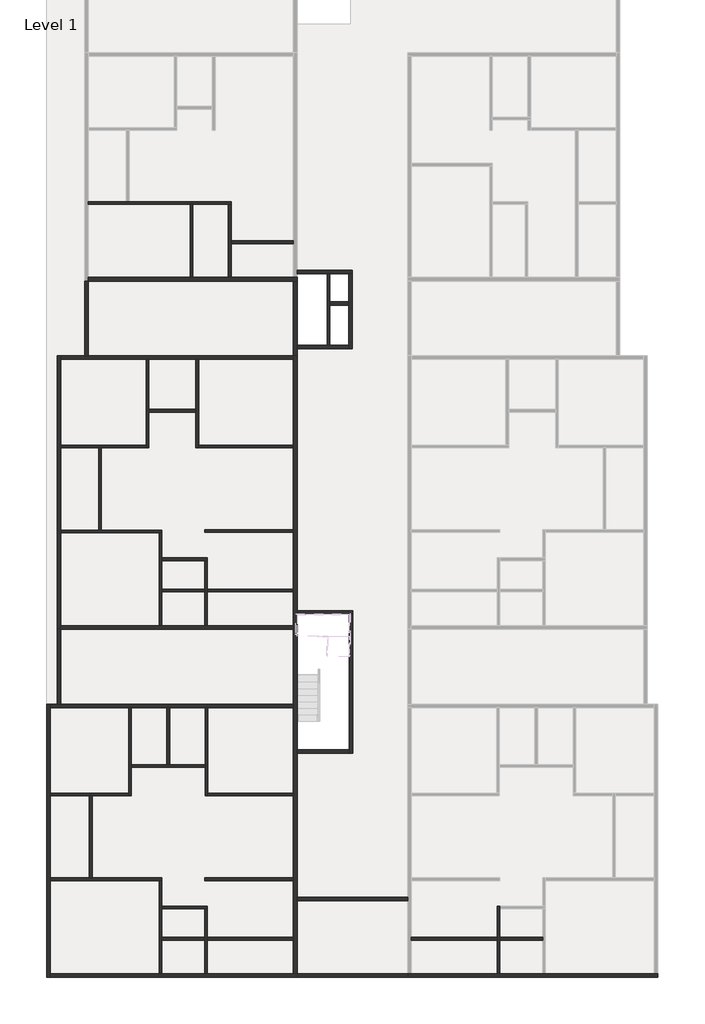
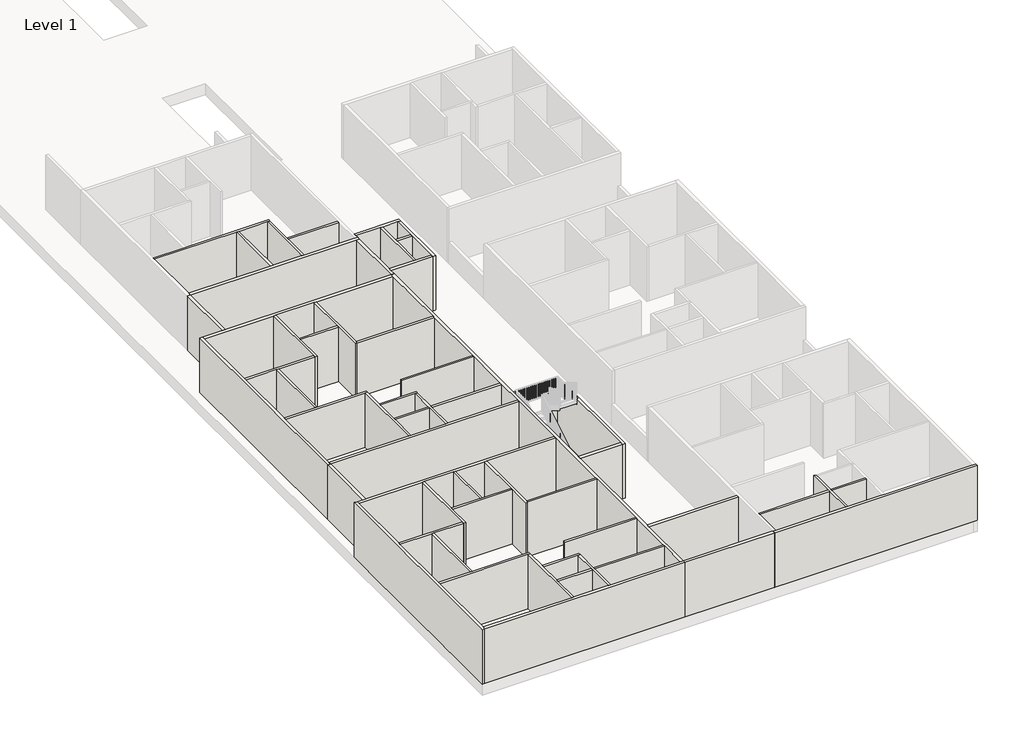
# One storey, part 1 of 8: 55 walls.
"""IFC4 building model written with IfcOpenShell, lengths in millimetres."""

from ifc_helpers import new_model, si_unit, frame, origin, place, context, project, spatial, polyline, outline, extrude, faceted_brep, element, save

model = new_model("IFC4")

# Units and contexts
model_context = context("Model", 3, world=origin())
ifc_project = project(units=[si_unit("LENGTHUNIT", "METRE", prefix="MILLI")], contexts=[model_context])

# Site, building, storey
site = spatial("IfcSite", under=ifc_project)
building = spatial("IfcBuilding", under=site)
storey = spatial("IfcBuildingStorey", under=building, Name="Level 1", Elevation=25234.6172466)

# Walls
placement = place(None, origin())
element("IfcWall", 1, ObjectType="4.5\"", at=placement, inside=storey, context=model_context, shape_type="Brep", body=[
    faceted_brep([(-12531.5544854, -1061.7344126, 25234.6172466), (-8188.1544854, -1061.7344126, 25234.6172466), (-8073.8544854, -1061.7344126, 25234.6172466), (-6549.8544854, -1061.7344126, 25234.6172466), (-6435.5544854, -1061.7344126, 25234.6172466), (-6435.5544854, -1061.7344126, 28282.6172466), (-6549.8544854, -1061.7344126, 28282.6172466), (-8073.8544854, -1061.7344126, 28282.6172466), (-8188.1544854, -1061.7344126, 28282.6172466), (-12531.5544854, -1061.7344126, 28282.6172466), (-12531.5544854, -947.4344126, 25234.6172466), (-12531.5544854, -947.4344126, 28282.6172466), (-10907.2415084, -947.4344126, 28282.6172466), (-10792.9415084, -947.4344126, 28282.6172466), (-6435.5544854, -947.4344126, 28282.6172466), (-6435.5544854, -947.4344126, 25234.6172466), (-10792.9415084, -947.4344126, 25234.6172466), (-10907.2415084, -947.4344126, 25234.6172466)], [[[0, 1, 2, 3, 4, 5, 6, 7, 8, 9]], [[10, 11, 12, 13, 14, 15, 16, 17]], [[4, 3, 2, 1, 0, 10, 17, 16, 15]], [[0, 9, 11, 10]], [[5, 4, 15, 14]], [[9, 8, 7, 6, 5, 14, 13, 12, 11]]]),
])
element("IfcWall", 2, ObjectType="4.5\"", at=placement, inside=storey, context=model_context, shape_type="Brep", body=[
    faceted_brep([(-6549.8544854, -1061.7344126, 25234.6172466), (-6549.8544854, -4185.9344126, 25234.6172466), (-6549.8544854, -4185.9344126, 28282.6172466), (-6549.8544854, -1061.7344126, 28282.6172466), (-6435.5544854, -1061.7344126, 25234.6172466), (-6435.5544854, -1061.7344126, 28282.6172466), (-6435.5544854, -2623.8344126, 28282.6172466), (-6435.5544854, -2738.1344126, 28282.6172466), (-6435.5544854, -4185.9344126, 28282.6172466), (-6435.5544854, -4185.9344126, 25234.6172466), (-6435.5544854, -2738.1344126, 25234.6172466), (-6435.5544854, -2623.8344126, 25234.6172466)], [[[0, 1, 2, 3]], [[4, 5, 6, 7, 8, 9, 10, 11]], [[1, 0, 4, 11, 10, 9]], [[0, 3, 5, 4]], [[2, 1, 9, 8]], [[3, 2, 8, 7, 6, 5]]]),
])
element("IfcWall", 3, ObjectType="4.5\"", at=placement, inside=storey, context=model_context, shape_type="SweptSolid", body=[
    extrude(outline(polyline([(-8188.1544854, -4185.9344126), (-8188.1544854, -1061.7344126), (-8073.8544854, -1061.7344126), (-8073.8544854, -4185.9344126), (-8188.1544854, -4185.9344126)])), frame((0.0, 0.0, 25234.6172466), z_axis=(0.0, 0.0, 1.0), x_axis=(1.0, 0.0, 0.0)), (0.0, 0.0, 1.0), 3048.0),
])
element("IfcWall", 4, ObjectType="4.5\"", at=placement, inside=storey, context=model_context, shape_type="SweptSolid", body=[
    extrude(outline(polyline([(-6435.5544854, -2623.8344126), (-3769.8415084, -2623.8344126), (-3769.8415084, -2738.1344126), (-6435.5544854, -2738.1344126), (-6435.5544854, -2623.8344126)])), frame((0.0, 0.0, 25234.6172466), z_axis=(0.0, 0.0, 1.0), x_axis=(1.0, 0.0, 0.0)), (0.0, 0.0, 1.0), 3048.0),
])
element("IfcWall", 5, ObjectType="4.5\"", at=placement, inside=storey, context=model_context, shape_type="Brep", body=[
    faceted_brep([(-10061.4044854, -7691.1344126, 25234.6172466), (-10061.4044854, -11348.7344126, 25234.6172466), (-10061.4044854, -11463.0344126, 25234.6172466), (-10061.4044854, -11463.0344126, 28282.6172466), (-10061.4044854, -11348.7344126, 28282.6172466), (-10061.4044854, -7691.1344126, 28282.6172466), (-9947.1044854, -7691.1344126, 25234.6172466), (-9947.1044854, -7691.1344126, 28282.6172466), (-9947.1044854, -9824.7344126, 28282.6172466), (-9947.1044854, -9939.0344126, 28282.6172466), (-9947.1044854, -11463.0344126, 28282.6172466), (-9947.1044854, -11463.0344126, 25234.6172466), (-9947.1044854, -9939.0344126, 25234.6172466), (-9947.1044854, -9824.7344126, 25234.6172466)], [[[0, 1, 2, 3, 4, 5]], [[6, 7, 8, 9, 10, 11, 12, 13]], [[2, 1, 0, 6, 13, 12, 11]], [[0, 5, 7, 6]], [[3, 2, 11, 10]], [[5, 4, 3, 10, 9, 8, 7]]]),
])
element("IfcWall", 6, ObjectType="4.5\"", at=placement, inside=storey, context=model_context, shape_type="Brep", body=[
    faceted_brep([(-10061.4044854, -11348.7344126, 25234.6172466), (-13719.0044854, -11348.7344126, 25234.6172466), (-13719.0044854, -11348.7344126, 28282.6172466), (-10061.4044854, -11348.7344126, 28282.6172466), (-10061.4044854, -11463.0344126, 25234.6172466), (-10061.4044854, -11463.0344126, 28282.6172466), (-11980.3915084, -11463.0344126, 28282.6172466), (-12094.6915084, -11463.0344126, 28282.6172466), (-13719.0044854, -11463.0344126, 28282.6172466), (-13719.0044854, -11463.0344126, 25234.6172466), (-12094.6915084, -11463.0344126, 25234.6172466), (-11980.3915084, -11463.0344126, 25234.6172466)], [[[0, 1, 2, 3]], [[4, 5, 6, 7, 8, 9, 10, 11]], [[1, 0, 4, 11, 10, 9]], [[0, 3, 5, 4]], [[2, 1, 9, 8]], [[3, 2, 8, 7, 6, 5]]]),
])
element("IfcWall", 7, ObjectType="4.5\"", at=placement, inside=storey, context=model_context, shape_type="SweptSolid", body=[
    extrude(outline(polyline([(-12094.6915084, -14968.2344126), (-12094.6915084, -11463.0344126), (-11980.3915084, -11463.0344126), (-11980.3915084, -14968.2344126), (-12094.6915084, -14968.2344126)])), frame((0.0, 0.0, 25234.6172466), z_axis=(0.0, 0.0, 1.0), x_axis=(1.0, 0.0, 0.0)), (0.0, 0.0, 1.0), 3048.0),
])
element("IfcWall", 8, ObjectType="4.5\"", at=placement, inside=storey, context=model_context, shape_type="Brep", body=[
    faceted_brep([(-13719.0044854, -15095.2344126, 25234.6172466), (-9510.2415084, -15095.2344126, 25234.6172466), (-9395.9415084, -15095.2344126, 25234.6172466), (-9395.9415084, -15095.2344126, 28282.6172466), (-9510.2415084, -15095.2344126, 28282.6172466), (-13719.0044854, -15095.2344126, 28282.6172466), (-13719.0044854, -14980.9344126, 25234.6172466), (-13719.0044854, -14980.9344126, 28282.6172466), (-9395.9415084, -14980.9344126, 28282.6172466), (-9395.9415084, -14980.9344126, 25234.6172466)], [[[0, 1, 2, 3, 4, 5]], [[6, 7, 8, 9]], [[2, 1, 0, 6, 9]], [[0, 5, 7, 6]], [[3, 2, 9, 8]], [[5, 4, 3, 8, 7]]]),
])
element("IfcWall", 9, ObjectType="4.5\"", at=placement, inside=storey, context=model_context, shape_type="Brep", body=[
    faceted_brep([(-9510.2415084, -15095.2344126, 25234.6172466), (-9510.2415084, -19070.3344126, 25234.6172466), (-9510.2415084, -19070.3344126, 28282.6172466), (-9510.2415084, -15095.2344126, 28282.6172466), (-9395.9415084, -15095.2344126, 25234.6172466), (-9395.9415084, -15095.2344126, 28282.6172466), (-9395.9415084, -16174.7344126, 28282.6172466), (-9395.9415084, -16289.0344126, 28282.6172466), (-9395.9415084, -17508.2344126, 28282.6172466), (-9395.9415084, -17622.5344126, 28282.6172466), (-9395.9415084, -19070.3344126, 28282.6172466), (-9395.9415084, -19070.3344126, 25234.6172466), (-9395.9415084, -17622.5344126, 25234.6172466), (-9395.9415084, -17508.2344126, 25234.6172466), (-9395.9415084, -16289.0344126, 25234.6172466), (-9395.9415084, -16174.7344126, 25234.6172466)], [[[0, 1, 2, 3]], [[4, 5, 6, 7, 8, 9, 10, 11, 12, 13, 14, 15]], [[1, 0, 4, 15, 14, 13, 12, 11]], [[0, 3, 5, 4]], [[2, 1, 11, 10]], [[3, 2, 10, 9, 8, 7, 6, 5]]]),
])
element("IfcWall", 10, ObjectType="4.5\"", at=placement, inside=storey, context=model_context, shape_type="Brep", body=[
    faceted_brep([(-9395.9415084, -16289.0344126, 25234.6172466), (-7567.1415084, -16289.0344126, 25234.6172466), (-7452.8415084, -16289.0344126, 25234.6172466), (-7452.8415084, -16289.0344126, 28282.6172466), (-7567.1415084, -16289.0344126, 28282.6172466), (-9395.9415084, -16289.0344126, 28282.6172466), (-9395.9415084, -16174.7344126, 25234.6172466), (-9395.9415084, -16174.7344126, 28282.6172466), (-7452.8415084, -16174.7344126, 28282.6172466), (-7452.8415084, -16174.7344126, 25234.6172466)], [[[0, 1, 2, 3, 4, 5]], [[6, 7, 8, 9]], [[2, 1, 0, 6, 9]], [[0, 5, 7, 6]], [[3, 2, 9, 8]], [[5, 4, 3, 8, 7]]]),
])
element("IfcWall", 11, ObjectType="4.5\"", at=placement, inside=storey, context=model_context, shape_type="Brep", body=[
    faceted_brep([(-7567.1415084, -16289.0344126, 25234.6172466), (-7567.1415084, -17508.2344126, 25234.6172466), (-7567.1415084, -17622.5344126, 25234.6172466), (-7567.1415084, -19070.3344126, 25234.6172466), (-7567.1415084, -19070.3344126, 28282.6172466), (-7567.1415084, -17622.5344126, 28282.6172466), (-7567.1415084, -17508.2344126, 28282.6172466), (-7567.1415084, -16289.0344126, 28282.6172466), (-7452.8415084, -16289.0344126, 25234.6172466), (-7452.8415084, -16289.0344126, 28282.6172466), (-7452.8415084, -17508.2344126, 28282.6172466), (-7452.8415084, -17622.5344126, 28282.6172466), (-7452.8415084, -19070.3344126, 28282.6172466), (-7452.8415084, -19070.3344126, 25234.6172466), (-7452.8415084, -17622.5344126, 25234.6172466), (-7452.8415084, -17508.2344126, 25234.6172466)], [[[0, 1, 2, 3, 4, 5, 6, 7]], [[8, 9, 10, 11, 12, 13, 14, 15]], [[3, 2, 1, 0, 8, 15, 14, 13]], [[0, 7, 9, 8]], [[4, 3, 13, 12]], [[7, 6, 5, 4, 12, 11, 10, 9]]]),
])
element("IfcWall", 12, ObjectType="4.5\"", at=placement, inside=storey, context=model_context, shape_type="SweptSolid", body=[
    extrude(outline(polyline([(-7567.1415084, -17622.5344126), (-9395.9415084, -17622.5344126), (-9395.9415084, -17508.2344126), (-7567.1415084, -17508.2344126), (-7567.1415084, -17622.5344126)])), frame((0.0, 0.0, 25234.6172466), z_axis=(0.0, 0.0, 1.0), x_axis=(1.0, 0.0, 0.0)), (0.0, 0.0, 1.0), 3048.0),
])
element("IfcWall", 13, ObjectType="4.5\"", at=placement, inside=storey, context=model_context, shape_type="SweptSolid", body=[
    extrude(outline(polyline([(-3769.8415084, -17622.5344126), (-7452.8415084, -17622.5344126), (-7452.8415084, -17508.2344126), (-3769.8415084, -17508.2344126), (-3769.8415084, -17622.5344126)])), frame((0.0, 0.0, 25234.6172466), z_axis=(0.0, 0.0, 1.0), x_axis=(1.0, 0.0, 0.0)), (0.0, 0.0, 1.0), 3048.0),
])
element("IfcWall", 14, ObjectType="4.5\"", at=placement, inside=storey, context=model_context, shape_type="SweptSolid", body=[
    extrude(outline(polyline([(-7567.1415084, -14968.2344126), (-3769.8415084, -14968.2344126), (-3769.8415084, -15082.5344126), (-7567.1415084, -15082.5344126), (-7567.1415084, -14968.2344126)])), frame((0.0, 0.0, 25234.6172466), z_axis=(0.0, 0.0, 1.0), x_axis=(1.0, 0.0, 0.0)), (0.0, 0.0, 1.0), 3048.0),
])
element("IfcWall", 15, ObjectType="4.5\"", at=placement, inside=storey, context=model_context, shape_type="SweptSolid", body=[
    extrude(outline(polyline([(-7940.5044854, -9939.0344126), (-9947.1044854, -9939.0344126), (-9947.1044854, -9824.7344126), (-7940.5044854, -9824.7344126), (-7940.5044854, -9939.0344126)])), frame((0.0, 0.0, 25234.6172466), z_axis=(0.0, 0.0, 1.0), x_axis=(1.0, 0.0, 0.0)), (0.0, 0.0, 1.0), 3048.0),
])
element("IfcWall", 16, ObjectType="4.5\"", at=placement, inside=storey, context=model_context, shape_type="Brep", body=[
    faceted_brep([(-7940.5044854, -7691.1344126, 25234.6172466), (-7940.5044854, -9824.7344126, 25234.6172466), (-7940.5044854, -9939.0344126, 25234.6172466), (-7940.5044854, -11463.0344126, 25234.6172466), (-7940.5044854, -11463.0344126, 28282.6172466), (-7940.5044854, -9939.0344126, 28282.6172466), (-7940.5044854, -9824.7344126, 28282.6172466), (-7940.5044854, -7691.1344126, 28282.6172466), (-7826.2044854, -7691.1344126, 25234.6172466), (-7826.2044854, -7691.1344126, 28282.6172466), (-7826.2044854, -11348.7344126, 28282.6172466), (-7826.2044854, -11463.0344126, 28282.6172466), (-7826.2044854, -11463.0344126, 25234.6172466), (-7826.2044854, -11348.7344126, 25234.6172466)], [[[0, 1, 2, 3, 4, 5, 6, 7]], [[8, 9, 10, 11, 12, 13]], [[3, 2, 1, 0, 8, 13, 12]], [[0, 7, 9, 8]], [[4, 3, 12, 11]], [[7, 6, 5, 4, 11, 10, 9]]]),
])
element("IfcWall", 17, ObjectType="4.5\"", at=placement, inside=storey, context=model_context, shape_type="SweptSolid", body=[
    extrude(outline(polyline([(-3769.8415084, -11463.0344126), (-7826.2044854, -11463.0344126), (-7826.2044854, -11348.7344126), (-3769.8415084, -11348.7344126), (-3769.8415084, -11463.0344126)])), frame((0.0, 0.0, 25234.6172466), z_axis=(0.0, 0.0, 1.0), x_axis=(1.0, 0.0, 0.0)), (0.0, 0.0, 1.0), 3048.0),
])
element("IfcWall", 18, ObjectType="4.5\"", at=placement, inside=storey, context=model_context, shape_type="Brep", body=[
    faceted_brep([(-10818.3415084, -22575.5344126, 25234.6172466), (-10818.3415084, -26233.1344126, 25234.6172466), (-10818.3415084, -26347.4344126, 25234.6172466), (-10818.3415084, -26347.4344126, 28282.6172466), (-10818.3415084, -26233.1344126, 28282.6172466), (-10818.3415084, -22575.5344126, 28282.6172466), (-10704.0415084, -22575.5344126, 25234.6172466), (-10704.0415084, -22575.5344126, 28282.6172466), (-10704.0415084, -25013.9344126, 28282.6172466), (-10704.0415084, -25128.2344126, 28282.6172466), (-10704.0415084, -26347.4344126, 28282.6172466), (-10704.0415084, -26347.4344126, 25234.6172466), (-10704.0415084, -25128.2344126, 25234.6172466), (-10704.0415084, -25013.9344126, 25234.6172466)], [[[0, 1, 2, 3, 4, 5]], [[6, 7, 8, 9, 10, 11, 12, 13]], [[2, 1, 0, 6, 13, 12, 11]], [[0, 5, 7, 6]], [[3, 2, 11, 10]], [[5, 4, 3, 10, 9, 8, 7]]]),
])
element("IfcWall", 19, ObjectType="4.5\"", at=placement, inside=storey, context=model_context, shape_type="Brep", body=[
    faceted_brep([(-10818.3415084, -26233.1344126, 25234.6172466), (-14171.1415084, -26233.1344126, 25234.6172466), (-14171.1415084, -26233.1344126, 28282.6172466), (-10818.3415084, -26233.1344126, 28282.6172466), (-10818.3415084, -26347.4344126, 25234.6172466), (-10818.3415084, -26347.4344126, 28282.6172466), (-12380.4415084, -26347.4344126, 28282.6172466), (-12494.7415084, -26347.4344126, 28282.6172466), (-14171.1415084, -26347.4344126, 28282.6172466), (-14171.1415084, -26347.4344126, 25234.6172466), (-12494.7415084, -26347.4344126, 25234.6172466), (-12380.4415084, -26347.4344126, 25234.6172466)], [[[0, 1, 2, 3]], [[4, 5, 6, 7, 8, 9, 10, 11]], [[1, 0, 4, 11, 10, 9]], [[0, 3, 5, 4]], [[2, 1, 9, 8]], [[3, 2, 8, 7, 6, 5]]]),
])
element("IfcWall", 20, ObjectType="4.5\"", at=placement, inside=storey, context=model_context, shape_type="SweptSolid", body=[
    extrude(outline(polyline([(-9180.0415084, -25013.9344126), (-9180.0415084, -22575.5344126), (-9065.7415084, -22575.5344126), (-9065.7415084, -25013.9344126), (-9180.0415084, -25013.9344126)])), frame((0.0, 0.0, 25234.6172466), z_axis=(0.0, 0.0, 1.0), x_axis=(1.0, 0.0, 0.0)), (0.0, 0.0, 1.0), 3048.0),
])
element("IfcWall", 21, ObjectType="4.5\"", at=placement, inside=storey, context=model_context, shape_type="Brep", body=[
    faceted_brep([(-10704.0415084, -25128.2344126, 25234.6172466), (-7541.7415084, -25128.2344126, 25234.6172466), (-7541.7415084, -25128.2344126, 28282.6172466), (-10704.0415084, -25128.2344126, 28282.6172466), (-10704.0415084, -25013.9344126, 25234.6172466), (-10704.0415084, -25013.9344126, 28282.6172466), (-9180.0415084, -25013.9344126, 28282.6172466), (-9065.7415084, -25013.9344126, 28282.6172466), (-7541.7415084, -25013.9344126, 28282.6172466), (-7541.7415084, -25013.9344126, 25234.6172466), (-9065.7415084, -25013.9344126, 25234.6172466), (-9180.0415084, -25013.9344126, 25234.6172466)], [[[0, 1, 2, 3]], [[4, 5, 6, 7, 8, 9, 10, 11]], [[1, 0, 4, 11, 10, 9]], [[0, 3, 5, 4]], [[2, 1, 9, 8]], [[3, 2, 8, 7, 6, 5]]]),
])
element("IfcWall", 22, ObjectType="4.5\"", at=placement, inside=storey, context=model_context, shape_type="Brep", body=[
    faceted_brep([(-7541.7415084, -22575.5344126, 25234.6172466), (-7541.7415084, -25013.9344126, 25234.6172466), (-7541.7415084, -25128.2344126, 25234.6172466), (-7541.7415084, -26347.4344126, 25234.6172466), (-7541.7415084, -26347.4344126, 28282.6172466), (-7541.7415084, -25128.2344126, 28282.6172466), (-7541.7415084, -25013.9344126, 28282.6172466), (-7541.7415084, -22575.5344126, 28282.6172466), (-7427.4415084, -22575.5344126, 25234.6172466), (-7427.4415084, -22575.5344126, 28282.6172466), (-7427.4415084, -26233.1344126, 28282.6172466), (-7427.4415084, -26347.4344126, 28282.6172466), (-7427.4415084, -26347.4344126, 25234.6172466), (-7427.4415084, -26233.1344126, 25234.6172466)], [[[0, 1, 2, 3, 4, 5, 6, 7]], [[8, 9, 10, 11, 12, 13]], [[3, 2, 1, 0, 8, 13, 12]], [[0, 7, 9, 8]], [[4, 3, 12, 11]], [[7, 6, 5, 4, 11, 10, 9]]]),
])
element("IfcWall", 23, ObjectType="4.5\"", at=placement, inside=storey, context=model_context, shape_type="SweptSolid", body=[
    extrude(outline(polyline([(-3769.8415084, -26347.4344126), (-7427.4415084, -26347.4344126), (-7427.4415084, -26233.1344126), (-3769.8415084, -26233.1344126), (-3769.8415084, -26347.4344126)])), frame((0.0, 0.0, 25234.6172466), z_axis=(0.0, 0.0, 1.0), x_axis=(1.0, 0.0, 0.0)), (0.0, 0.0, 1.0), 3048.0),
])
element("IfcWall", 24, ObjectType="4.5\"", at=placement, inside=storey, context=model_context, shape_type="SweptSolid", body=[
    extrude(outline(polyline([(-12494.7415084, -29852.6344126), (-12494.7415084, -26347.4344126), (-12380.4415084, -26347.4344126), (-12380.4415084, -29852.6344126), (-12494.7415084, -29852.6344126)])), frame((0.0, 0.0, 25234.6172466), z_axis=(0.0, 0.0, 1.0), x_axis=(1.0, 0.0, 0.0)), (0.0, 0.0, 1.0), 3048.0),
])
element("IfcWall", 25, ObjectType="4.5\"", at=placement, inside=storey, context=model_context, shape_type="Brep", body=[
    faceted_brep([(-14171.1415084, -29966.9344126, 25234.6172466), (-9510.2415084, -29966.9344126, 25234.6172466), (-9395.9415084, -29966.9344126, 25234.6172466), (-9395.9415084, -29966.9344126, 28282.6172466), (-9510.2415084, -29966.9344126, 28282.6172466), (-14171.1415084, -29966.9344126, 28282.6172466), (-14171.1415084, -29852.6344126, 25234.6172466), (-14171.1415084, -29852.6344126, 28282.6172466), (-12494.7415084, -29852.6344126, 28282.6172466), (-12380.4415084, -29852.6344126, 28282.6172466), (-9395.9415084, -29852.6344126, 28282.6172466), (-9395.9415084, -29852.6344126, 25234.6172466), (-12380.4415084, -29852.6344126, 25234.6172466), (-12494.7415084, -29852.6344126, 25234.6172466)], [[[0, 1, 2, 3, 4, 5]], [[6, 7, 8, 9, 10, 11, 12, 13]], [[2, 1, 0, 6, 13, 12, 11]], [[0, 5, 7, 6]], [[3, 2, 11, 10]], [[5, 4, 3, 10, 9, 8, 7]]]),
])
element("IfcWall", 26, ObjectType="4.5\"", at=placement, inside=storey, context=model_context, shape_type="Brep", body=[
    faceted_brep([(-9510.2415084, -29966.9344126, 25234.6172466), (-9510.2415084, -33954.7344126, 25234.6172466), (-9510.2415084, -33954.7344126, 28282.6172466), (-9510.2415084, -29966.9344126, 28282.6172466), (-9395.9415084, -29966.9344126, 25234.6172466), (-9395.9415084, -29966.9344126, 28282.6172466), (-9395.9415084, -31059.1344126, 28282.6172466), (-9395.9415084, -31173.4344126, 28282.6172466), (-9395.9415084, -32392.6344126, 28282.6172466), (-9395.9415084, -32506.9344126, 28282.6172466), (-9395.9415084, -33954.7344126, 28282.6172466), (-9395.9415084, -33954.7344126, 25234.6172466), (-9395.9415084, -32506.9344126, 25234.6172466), (-9395.9415084, -32392.6344126, 25234.6172466), (-9395.9415084, -31173.4344126, 25234.6172466), (-9395.9415084, -31059.1344126, 25234.6172466)], [[[0, 1, 2, 3]], [[4, 5, 6, 7, 8, 9, 10, 11, 12, 13, 14, 15]], [[1, 0, 4, 15, 14, 13, 12, 11]], [[0, 3, 5, 4]], [[2, 1, 11, 10]], [[3, 2, 10, 9, 8, 7, 6, 5]]]),
])
element("IfcWall", 27, ObjectType="4.5\"", at=placement, inside=storey, context=model_context, shape_type="Brep", body=[
    faceted_brep([(-9395.9415084, -31173.4344126, 25234.6172466), (-7567.1415084, -31173.4344126, 25234.6172466), (-7452.8415084, -31173.4344126, 25234.6172466), (-7452.8415084, -31173.4344126, 28282.6172466), (-7567.1415084, -31173.4344126, 28282.6172466), (-9395.9415084, -31173.4344126, 28282.6172466), (-9395.9415084, -31059.1344126, 25234.6172466), (-9395.9415084, -31059.1344126, 28282.6172466), (-7452.8415084, -31059.1344126, 28282.6172466), (-7452.8415084, -31059.1344126, 25234.6172466)], [[[0, 1, 2, 3, 4, 5]], [[6, 7, 8, 9]], [[2, 1, 0, 6, 9]], [[0, 5, 7, 6]], [[3, 2, 9, 8]], [[5, 4, 3, 8, 7]]]),
])
element("IfcWall", 28, ObjectType="4.5\"", at=placement, inside=storey, context=model_context, shape_type="Brep", body=[
    faceted_brep([(-7567.1415084, -31173.4344126, 25234.6172466), (-7567.1415084, -32392.6344126, 25234.6172466), (-7567.1415084, -32506.9344126, 25234.6172466), (-7567.1415084, -33954.7344126, 25234.6172466), (-7567.1415084, -33954.7344126, 28282.6172466), (-7567.1415084, -32506.9344126, 28282.6172466), (-7567.1415084, -32392.6344126, 28282.6172466), (-7567.1415084, -31173.4344126, 28282.6172466), (-7452.8415084, -31173.4344126, 25234.6172466), (-7452.8415084, -31173.4344126, 28282.6172466), (-7452.8415084, -32392.6344126, 28282.6172466), (-7452.8415084, -32506.9344126, 28282.6172466), (-7452.8415084, -33954.7344126, 28282.6172466), (-7452.8415084, -33954.7344126, 25234.6172466), (-7452.8415084, -32506.9344126, 25234.6172466), (-7452.8415084, -32392.6344126, 25234.6172466)], [[[0, 1, 2, 3, 4, 5, 6, 7]], [[8, 9, 10, 11, 12, 13, 14, 15]], [[3, 2, 1, 0, 8, 15, 14, 13]], [[0, 7, 9, 8]], [[4, 3, 13, 12]], [[7, 6, 5, 4, 12, 11, 10, 9]]]),
])
element("IfcWall", 29, ObjectType="4.5\"", at=placement, inside=storey, context=model_context, shape_type="SweptSolid", body=[
    extrude(outline(polyline([(-3769.8415084, -32392.6344126), (-3769.8415084, -32506.9344126), (-7452.8415084, -32506.9344126), (-7452.8415084, -32392.6344126), (-3769.8415084, -32392.6344126)])), frame((0.0, 0.0, 25234.6172466), z_axis=(0.0, 0.0, 1.0), x_axis=(1.0, 0.0, 0.0)), (0.0, 0.0, 1.0), 3048.0),
    extrude(outline(polyline([(-9395.9415084, -32506.9344126), (-9395.9415084, -32392.6344126), (-7567.1415084, -32392.6344126), (-7567.1415084, -32506.9344126), (-9395.9415084, -32506.9344126)])), frame((0.0, 0.0, 25234.6172466), z_axis=(0.0, 0.0, 1.0), x_axis=(1.0, 0.0, 0.0)), (0.0, 0.0, 1.0), 3048.0),
])
element("IfcWall", 30, ObjectType="4.5\"", at=placement, inside=storey, context=model_context, shape_type="SweptSolid", body=[
    extrude(outline(polyline([(-7567.1415084, -29852.6344126), (-3769.8415084, -29852.6344126), (-3769.8415084, -29966.9344126), (-7567.1415084, -29966.9344126), (-7567.1415084, -29852.6344126)])), frame((0.0, 0.0, 25234.6172466), z_axis=(0.0, 0.0, 1.0), x_axis=(1.0, 0.0, 0.0)), (0.0, 0.0, 1.0), 3048.0),
])
element("IfcWall", 31, ObjectType="4.5\"", at=placement, inside=storey, context=model_context, shape_type="SweptSolid", body=[
    extrude(outline(polyline([(4942.3584916, -32506.9344126), (1259.3584916, -32506.9344126), (1259.3584916, -32392.6344126), (4942.3584916, -32392.6344126), (4942.3584916, -32506.9344126)])), frame((0.0, 0.0, 25234.6172466), z_axis=(0.0, 0.0, 1.0), x_axis=(1.0, 0.0, 0.0)), (0.0, 0.0, 1.0), 3048.0),
])
element("IfcWall", 32, ObjectType="4.5\"", at=placement, inside=storey, context=model_context, shape_type="Brep", body=[
    faceted_brep([(4942.3584916, -31059.1344126, 25234.6172466), (4942.3584916, -32392.6344126, 25234.6172466), (4942.3584916, -32506.9344126, 25234.6172466), (4942.3584916, -33954.7344126, 25234.6172466), (4942.3584916, -33954.7344126, 28282.6172466), (4942.3584916, -32506.9344126, 28282.6172466), (4942.3584916, -32392.6344126, 28282.6172466), (4942.3584916, -31059.1344126, 28282.6172466), (5056.6584916, -31059.1344126, 25234.6172466), (5056.6584916, -31059.1344126, 28282.6172466), (5056.6584916, -31173.4344126, 28282.6172466), (5056.6584916, -32392.6344126, 28282.6172466), (5056.6584916, -32506.9344126, 28282.6172466), (5056.6584916, -33954.7344126, 28282.6172466), (5056.6584916, -33954.7344126, 25234.6172466), (5056.6584916, -32506.9344126, 25234.6172466), (5056.6584916, -32392.6344126, 25234.6172466), (5056.6584916, -31173.4344126, 25234.6172466)], [[[0, 1, 2, 3, 4, 5, 6, 7]], [[8, 9, 10, 11, 12, 13, 14, 15, 16, 17]], [[3, 2, 1, 0, 8, 17, 16, 15, 14]], [[4, 3, 14, 13]], [[0, 7, 9, 8]], [[7, 6, 5, 4, 13, 12, 11, 10, 9]]]),
])
element("IfcWall", 33, ObjectType="4.5\"", at=placement, inside=storey, context=model_context, shape_type="SweptSolid", body=[
    extrude(outline(polyline([(6885.4584916, -32506.9344126), (5056.6584916, -32506.9344126), (5056.6584916, -32392.6344126), (6885.4584916, -32392.6344126), (6885.4584916, -32506.9344126)])), frame((0.0, 0.0, 25234.6172466), z_axis=(0.0, 0.0, 1.0), x_axis=(1.0, 0.0, 0.0)), (0.0, 0.0, 1.0), 3048.0),
])
element("IfcWall", 34, ObjectType="4.5\"", at=placement, inside=storey, context=model_context, shape_type="Brep", body=[
    faceted_brep([(-2207.6738684, -7082.6751812, 25234.6172466), (-2207.6738684, -5366.3479894, 25234.6172466), (-2207.6738684, -5213.9479894, 25234.6172466), (-2207.6738684, -4034.6751812, 25234.6172466), (-2207.6738684, -4034.6751812, 28282.6172466), (-2207.6738684, -5213.9479894, 28282.6172466), (-2207.6738684, -5366.3479894, 28282.6172466), (-2207.6738684, -7082.6751812, 28282.6172466), (-2321.9738684, -7082.6751812, 25234.6172466), (-2321.9738684, -7082.6751812, 28282.6172466), (-2321.9738684, -4034.6751812, 28282.6172466), (-2321.9738684, -4034.6751812, 25234.6172466)], [[[0, 1, 2, 3, 4, 5, 6, 7]], [[8, 9, 10, 11]], [[3, 2, 1, 0, 8, 11]], [[7, 6, 5, 4, 10, 9]], [[4, 3, 11, 10]], [[0, 7, 9, 8]]]),
])
element("IfcWall", 35, ObjectType="6\"", at=placement, inside=storey, context=model_context, shape_type="Brep", body=[
    faceted_brep([(-12531.5544854, -4338.3344126, 25234.6172466), (-3769.8415084, -4338.3344126, 25234.6172466), (-3617.4415084, -4338.3344126, 25234.6172466), (-3617.4415084, -4338.3344126, 28282.6172466), (-3769.8415084, -4338.3344126, 28282.6172466), (-12531.5544854, -4338.3344126, 28282.6172466), (-12531.5544854, -4185.9344126, 25234.6172466), (-12531.5544854, -4185.9344126, 28282.6172466), (-8188.1544854, -4185.9344126, 28282.6172466), (-8073.8544854, -4185.9344126, 28282.6172466), (-6549.8544854, -4185.9344126, 28282.6172466), (-6435.5544854, -4185.9344126, 28282.6172466), (-3769.8415084, -4185.9344126, 28282.6172466), (-3617.4415084, -4185.9344126, 28282.6172466), (-3617.4415084, -4185.9344126, 25234.6172466), (-3769.8415084, -4185.9344126, 25234.6172466), (-6435.5544854, -4185.9344126, 25234.6172466), (-6549.8544854, -4185.9344126, 25234.6172466), (-8073.8544854, -4185.9344126, 25234.6172466), (-8188.1544854, -4185.9344126, 25234.6172466)], [[[0, 1, 2, 3, 4, 5]], [[6, 7, 8, 9, 10, 11, 12, 13, 14, 15, 16, 17, 18, 19]], [[2, 1, 0, 6, 19, 18, 17, 16, 15, 14]], [[0, 5, 7, 6]], [[3, 2, 14, 13]], [[5, 4, 3, 13, 12, 11, 10, 9, 8, 7]]]),
])
element("IfcWall", 36, ObjectType="6\"", at=placement, inside=storey, context=model_context, shape_type="Brep", body=[
    faceted_brep([(-13871.4044854, -7538.7344126, 25234.6172466), (-13871.4044854, -19222.7344126, 25234.6172466), (-13871.4044854, -19222.7344126, 28282.6172466), (-13871.4044854, -7538.7344126, 28282.6172466), (-13719.0044854, -7538.7344126, 25234.6172466), (-13719.0044854, -7538.7344126, 28282.6172466), (-13719.0044854, -7691.1344126, 28282.6172466), (-13719.0044854, -11348.7344126, 28282.6172466), (-13719.0044854, -11463.0344126, 28282.6172466), (-13719.0044854, -14980.9344126, 28282.6172466), (-13719.0044854, -15095.2344126, 28282.6172466), (-13719.0044854, -19070.3344126, 28282.6172466), (-13719.0044854, -19222.7344126, 28282.6172466), (-13719.0044854, -19222.7344126, 25234.6172466), (-13719.0044854, -19070.3344126, 25234.6172466), (-13719.0044854, -15095.2344126, 25234.6172466), (-13719.0044854, -14980.9344126, 25234.6172466), (-13719.0044854, -11463.0344126, 25234.6172466), (-13719.0044854, -11348.7344126, 25234.6172466), (-13719.0044854, -7691.1344126, 25234.6172466)], [[[0, 1, 2, 3]], [[4, 5, 6, 7, 8, 9, 10, 11, 12, 13, 14, 15, 16, 17, 18, 19]], [[1, 0, 4, 19, 18, 17, 16, 15, 14, 13]], [[2, 1, 13, 12]], [[0, 3, 5, 4]], [[3, 2, 12, 11, 10, 9, 8, 7, 6, 5]]]),
])
element("IfcWall", 37, ObjectType="6\"", at=placement, inside=storey, context=model_context, shape_type="Brep", body=[
    faceted_brep([(-13719.0044854, -19222.7344126, 25234.6172466), (-3769.8415084, -19222.7344126, 25234.6172466), (-3769.8415084, -19222.7344126, 28282.6172466), (-13719.0044854, -19222.7344126, 28282.6172466), (-13719.0044854, -19070.3344126, 25234.6172466), (-13719.0044854, -19070.3344126, 28282.6172466), (-9510.2415084, -19070.3344126, 28282.6172466), (-9395.9415084, -19070.3344126, 28282.6172466), (-7567.1415084, -19070.3344126, 28282.6172466), (-7452.8415084, -19070.3344126, 28282.6172466), (-3769.8415084, -19070.3344126, 28282.6172466), (-3769.8415084, -19070.3344126, 25234.6172466), (-7452.8415084, -19070.3344126, 25234.6172466), (-7567.1415084, -19070.3344126, 25234.6172466), (-9395.9415084, -19070.3344126, 25234.6172466), (-9510.2415084, -19070.3344126, 25234.6172466)], [[[0, 1, 2, 3]], [[4, 5, 6, 7, 8, 9, 10, 11, 12, 13, 14, 15]], [[1, 0, 4, 15, 14, 13, 12, 11]], [[0, 3, 5, 4]], [[2, 1, 11, 10]], [[3, 2, 10, 9, 8, 7, 6, 5]]]),
])
element("IfcWall", 38, ObjectType="6\"", at=placement, inside=storey, context=model_context, shape_type="Brep", body=[
    faceted_brep([(-3617.4415084, -33954.7344126, 25234.6172466), (-3617.4415084, -30820.9325185, 25234.6172466), (-3617.4415084, -30668.5325185, 25234.6172466), (-3617.4415084, -24525.9851539, 25234.6172466), (-3617.4415084, -24373.5851539, 25234.6172466), (-3617.4415084, -18582.3851539, 25234.6172466), (-3617.4415084, -18429.9851539, 25234.6172466), (-3617.4415084, -7538.7344126, 25234.6172466), (-3617.4415084, -7538.7344126, 28282.6172466), (-3617.4415084, -18429.9851539, 28282.6172466), (-3617.4415084, -18582.3851539, 28282.6172466), (-3617.4415084, -24373.5851539, 28282.6172466), (-3617.4415084, -24525.9851539, 28282.6172466), (-3617.4415084, -30668.5325185, 28282.6172466), (-3617.4415084, -30820.9325185, 28282.6172466), (-3617.4415084, -33954.7344126, 28282.6172466), (-3769.8415084, -33954.7344126, 25234.6172466), (-3769.8415084, -33954.7344126, 28282.6172466), (-3769.8415084, -32506.9344126, 28282.6172466), (-3769.8415084, -32392.6344126, 28282.6172466), (-3769.8415084, -29966.9344126, 28282.6172466), (-3769.8415084, -29852.6344126, 28282.6172466), (-3769.8415084, -26347.4344126, 28282.6172466), (-3769.8415084, -26233.1344126, 28282.6172466), (-3769.8415084, -22575.5344126, 28282.6172466), (-3769.8415084, -22423.1344126, 28282.6172466), (-3769.8415084, -19222.7344126, 28282.6172466), (-3769.8415084, -19070.3344126, 28282.6172466), (-3769.8415084, -17622.5344126, 28282.6172466), (-3769.8415084, -17508.2344126, 28282.6172466), (-3769.8415084, -15082.5344126, 28282.6172466), (-3769.8415084, -14968.2344126, 28282.6172466), (-3769.8415084, -11463.0344126, 28282.6172466), (-3769.8415084, -11348.7344126, 28282.6172466), (-3769.8415084, -7691.1344126, 28282.6172466), (-3769.8415084, -7538.7344126, 28282.6172466), (-3769.8415084, -7538.7344126, 25234.6172466), (-3769.8415084, -7691.1344126, 25234.6172466), (-3769.8415084, -11348.7344126, 25234.6172466), (-3769.8415084, -11463.0344126, 25234.6172466), (-3769.8415084, -14968.2344126, 25234.6172466), (-3769.8415084, -15082.5344126, 25234.6172466), (-3769.8415084, -17508.2344126, 25234.6172466), (-3769.8415084, -17622.5344126, 25234.6172466), (-3769.8415084, -19070.3344126, 25234.6172466), (-3769.8415084, -19222.7344126, 25234.6172466), (-3769.8415084, -22423.1344126, 25234.6172466), (-3769.8415084, -22575.5344126, 25234.6172466), (-3769.8415084, -26233.1344126, 25234.6172466), (-3769.8415084, -26347.4344126, 25234.6172466), (-3769.8415084, -29852.6344126, 25234.6172466), (-3769.8415084, -29966.9344126, 25234.6172466), (-3769.8415084, -32392.6344126, 25234.6172466), (-3769.8415084, -32506.9344126, 25234.6172466)], [[[0, 1, 2, 3, 4, 5, 6, 7, 8, 9, 10, 11, 12, 13, 14, 15]], [[16, 17, 18, 19, 20, 21, 22, 23, 24, 25, 26, 27, 28, 29, 30, 31, 32, 33, 34, 35, 36, 37, 38, 39, 40, 41, 42, 43, 44, 45, 46, 47, 48, 49, 50, 51, 52, 53]], [[7, 6, 5, 4, 3, 2, 1, 0, 16, 53, 52, 51, 50, 49, 48, 47, 46, 45, 44, 43, 42, 41, 40, 39, 38, 37, 36]], [[8, 7, 36, 35]], [[0, 15, 17, 16]], [[15, 14, 13, 12, 11, 10, 9, 8, 35, 34, 33, 32, 31, 30, 29, 28, 27, 26, 25, 24, 23, 22, 21, 20, 19, 18, 17]]]),
])
element("IfcWall", 39, ObjectType="6\"", at=placement, inside=storey, context=model_context, shape_type="Brep", body=[
    faceted_brep([(-3769.8415084, -7538.7344126, 25234.6172466), (-12531.5544854, -7538.7344126, 25234.6172466), (-12683.9544854, -7538.7344126, 25234.6172466), (-13719.0044854, -7538.7344126, 25234.6172466), (-13719.0044854, -7538.7344126, 28282.6172466), (-12683.9544854, -7538.7344126, 28282.6172466), (-12531.5544854, -7538.7344126, 28282.6172466), (-3769.8415084, -7538.7344126, 28282.6172466), (-3769.8415084, -7691.1344126, 25234.6172466), (-3769.8415084, -7691.1344126, 28282.6172466), (-7826.2044854, -7691.1344126, 28282.6172466), (-7940.5044854, -7691.1344126, 28282.6172466), (-9947.1044854, -7691.1344126, 28282.6172466), (-10061.4044854, -7691.1344126, 28282.6172466), (-13719.0044854, -7691.1344126, 28282.6172466), (-13719.0044854, -7691.1344126, 25234.6172466), (-10061.4044854, -7691.1344126, 25234.6172466), (-9947.1044854, -7691.1344126, 25234.6172466), (-7940.5044854, -7691.1344126, 25234.6172466), (-7826.2044854, -7691.1344126, 25234.6172466)], [[[0, 1, 2, 3, 4, 5, 6, 7]], [[8, 9, 10, 11, 12, 13, 14, 15, 16, 17, 18, 19]], [[3, 2, 1, 0, 8, 19, 18, 17, 16, 15]], [[0, 7, 9, 8]], [[4, 3, 15, 14]], [[7, 6, 5, 4, 14, 13, 12, 11, 10, 9]]]),
])
element("IfcWall", 40, ObjectType="6\"", at=placement, inside=storey, context=model_context, shape_type="Brep", body=[
    faceted_brep([(-14323.5415084, -22423.1344126, 25234.6172466), (-14323.5415084, -34107.1344126, 25234.6172466), (-14323.5415084, -34107.1344126, 28282.6172466), (-14323.5415084, -22423.1344126, 28282.6172466), (-14171.1415084, -22423.1344126, 25234.6172466), (-14171.1415084, -22423.1344126, 28282.6172466), (-14171.1415084, -22575.5344126, 28282.6172466), (-14171.1415084, -26233.1344126, 28282.6172466), (-14171.1415084, -26347.4344126, 28282.6172466), (-14171.1415084, -29852.6344126, 28282.6172466), (-14171.1415084, -29966.9344126, 28282.6172466), (-14171.1415084, -33954.7344126, 28282.6172466), (-14171.1415084, -34107.1344126, 28282.6172466), (-14171.1415084, -34107.1344126, 25234.6172466), (-14171.1415084, -33954.7344126, 25234.6172466), (-14171.1415084, -29966.9344126, 25234.6172466), (-14171.1415084, -29852.6344126, 25234.6172466), (-14171.1415084, -26347.4344126, 25234.6172466), (-14171.1415084, -26233.1344126, 25234.6172466), (-14171.1415084, -22575.5344126, 25234.6172466)], [[[0, 1, 2, 3]], [[4, 5, 6, 7, 8, 9, 10, 11, 12, 13, 14, 15, 16, 17, 18, 19]], [[1, 0, 4, 19, 18, 17, 16, 15, 14, 13]], [[2, 1, 13, 12]], [[0, 3, 5, 4]], [[3, 2, 12, 11, 10, 9, 8, 7, 6, 5]]]),
])
element("IfcWall", 41, ObjectType="6\"", at=placement, inside=storey, context=model_context, shape_type="Brep", body=[
    faceted_brep([(-14171.1415084, -34107.1344126, 25234.6172466), (-3617.4415084, -34107.1344126, 25234.6172466), (-3617.4415084, -34107.1344126, 28282.6172466), (-14171.1415084, -34107.1344126, 28282.6172466), (-14171.1415084, -33954.7344126, 25234.6172466), (-14171.1415084, -33954.7344126, 28282.6172466), (-9510.2415084, -33954.7344126, 28282.6172466), (-9395.9415084, -33954.7344126, 28282.6172466), (-7567.1415084, -33954.7344126, 28282.6172466), (-7452.8415084, -33954.7344126, 28282.6172466), (-3769.8415084, -33954.7344126, 28282.6172466), (-3617.4415084, -33954.7344126, 28282.6172466), (-3617.4415084, -33954.7344126, 25234.6172466), (-3769.8415084, -33954.7344126, 25234.6172466), (-7452.8415084, -33954.7344126, 25234.6172466), (-7567.1415084, -33954.7344126, 25234.6172466), (-9395.9415084, -33954.7344126, 25234.6172466), (-9510.2415084, -33954.7344126, 25234.6172466)], [[[0, 1, 2, 3]], [[4, 5, 6, 7, 8, 9, 10, 11, 12, 13, 14, 15, 16, 17]], [[1, 0, 4, 17, 16, 15, 14, 13, 12]], [[0, 3, 5, 4]], [[2, 1, 12, 11]], [[3, 2, 11, 10, 9, 8, 7, 6, 5]]]),
])
element("IfcWall", 42, ObjectType="6\"", at=placement, inside=storey, context=model_context, shape_type="Brep", body=[
    faceted_brep([(-3769.8415084, -22423.1344126, 25234.6172466), (-13719.0044854, -22423.1344126, 25234.6172466), (-13871.4044854, -22423.1344126, 25234.6172466), (-14171.1415084, -22423.1344126, 25234.6172466), (-14171.1415084, -22423.1344126, 28282.6172466), (-13871.4044854, -22423.1344126, 28282.6172466), (-13719.0044854, -22423.1344126, 28282.6172466), (-3769.8415084, -22423.1344126, 28282.6172466), (-3769.8415084, -22575.5344126, 25234.6172466), (-3769.8415084, -22575.5344126, 28282.6172466), (-7427.4415084, -22575.5344126, 28282.6172466), (-7541.7415084, -22575.5344126, 28282.6172466), (-9065.7415084, -22575.5344126, 28282.6172466), (-9180.0415084, -22575.5344126, 28282.6172466), (-10704.0415084, -22575.5344126, 28282.6172466), (-10818.3415084, -22575.5344126, 28282.6172466), (-14171.1415084, -22575.5344126, 28282.6172466), (-14171.1415084, -22575.5344126, 25234.6172466), (-10818.3415084, -22575.5344126, 25234.6172466), (-10704.0415084, -22575.5344126, 25234.6172466), (-9180.0415084, -22575.5344126, 25234.6172466), (-9065.7415084, -22575.5344126, 25234.6172466), (-7541.7415084, -22575.5344126, 25234.6172466), (-7427.4415084, -22575.5344126, 25234.6172466)], [[[0, 1, 2, 3, 4, 5, 6, 7]], [[8, 9, 10, 11, 12, 13, 14, 15, 16, 17, 18, 19, 20, 21, 22, 23]], [[3, 2, 1, 0, 8, 23, 22, 21, 20, 19, 18, 17]], [[0, 7, 9, 8]], [[4, 3, 17, 16]], [[7, 6, 5, 4, 16, 15, 14, 13, 12, 11, 10, 9]]]),
])
element("IfcWall", 43, ObjectType="6\"", at=placement, inside=storey, context=model_context, shape_type="Brep", body=[
    faceted_brep([(1106.9584916, -34107.1344126, 25234.6172466), (11813.0584916, -34107.1344126, 25234.6172466), (11813.0584916, -34107.1344126, 28282.6172466), (1106.9584916, -34107.1344126, 28282.6172466), (1106.9584916, -33954.7344126, 25234.6172466), (1106.9584916, -33954.7344126, 28282.6172466), (1259.3584916, -33954.7344126, 28282.6172466), (4942.3584916, -33954.7344126, 28282.6172466), (5056.6584916, -33954.7344126, 28282.6172466), (6885.4584916, -33954.7344126, 28282.6172466), (6999.7584916, -33954.7344126, 28282.6172466), (11660.6584916, -33954.7344126, 28282.6172466), (11813.0584916, -33954.7344126, 28282.6172466), (11813.0584916, -33954.7344126, 25234.6172466), (11660.6584916, -33954.7344126, 25234.6172466), (6999.7584916, -33954.7344126, 25234.6172466), (6885.4584916, -33954.7344126, 25234.6172466), (5056.6584916, -33954.7344126, 25234.6172466), (4942.3584916, -33954.7344126, 25234.6172466), (1259.3584916, -33954.7344126, 25234.6172466)], [[[0, 1, 2, 3]], [[4, 5, 6, 7, 8, 9, 10, 11, 12, 13, 14, 15, 16, 17, 18, 19]], [[1, 0, 4, 19, 18, 17, 16, 15, 14, 13]], [[2, 1, 13, 12]], [[0, 3, 5, 4]], [[3, 2, 12, 11, 10, 9, 8, 7, 6, 5]]]),
])
element("IfcWall", 44, ObjectType="6\"", at=placement, inside=storey, context=model_context, shape_type="Brep", body=[
    faceted_brep([(-3617.4415084, -18582.3851539, 25234.6172466), (-1382.2415084, -18582.3851539, 25234.6172466), (-1229.8415084, -18582.3851539, 25234.6172466), (-1229.8415084, -18582.3851539, 28282.6172466), (-1382.2415084, -18582.3851539, 28282.6172466), (-3617.4415084, -18582.3851539, 28282.6172466), (-3617.4415084, -18429.9851539, 25234.6172466), (-3617.4415084, -18429.9851539, 28282.6172466), (-1229.8415084, -18429.9851539, 28282.6172466), (-1229.8415084, -18429.9851539, 25234.6172466)], [[[0, 1, 2, 3, 4, 5]], [[6, 7, 8, 9]], [[2, 1, 0, 6, 9]], [[5, 4, 3, 8, 7]], [[0, 5, 7, 6]], [[3, 2, 9, 8]]]),
])
element("IfcWall", 45, ObjectType="6\"", at=placement, inside=storey, context=model_context, shape_type="Brep", body=[
    faceted_brep([(-1382.2415084, -18582.3851539, 25234.6172466), (-1382.2415084, -24373.5851539, 25234.6172466), (-1382.2415084, -24525.9851539, 25234.6172466), (-1382.2415084, -24525.9851539, 28282.6172466), (-1382.2415084, -24373.5851539, 28282.6172466), (-1382.2415084, -18582.3851539, 28282.6172466), (-1229.8415084, -18582.3851539, 25234.6172466), (-1229.8415084, -18582.3851539, 28282.6172466), (-1229.8415084, -24525.9851539, 28282.6172466), (-1229.8415084, -24525.9851539, 25234.6172466)], [[[0, 1, 2, 3, 4, 5]], [[6, 7, 8, 9]], [[2, 1, 0, 6, 9]], [[5, 4, 3, 8, 7]], [[0, 5, 7, 6]], [[3, 2, 9, 8]]]),
])
element("IfcWall", 46, ObjectType="6\"", at=placement, inside=storey, context=model_context, shape_type="SweptSolid", body=[
    extrude(outline(polyline([(-3617.4415084, -24373.5851539), (-1382.2415084, -24373.5851539), (-1382.2415084, -24525.9851539), (-3617.4415084, -24525.9851539), (-3617.4415084, -24373.5851539)])), frame((0.0, 0.0, 25234.6172466), z_axis=(0.0, 0.0, 1.0), x_axis=(1.0, 0.0, 0.0)), (0.0, 0.0, 1.0), 3048.0),
])
element("IfcWall", 47, ObjectType="6\"", at=placement, inside=storey, context=model_context, shape_type="Brep", body=[
    faceted_brep([(-3769.8415084, -4338.3344126, 25234.6172466), (-3769.8415084, -7538.7344126, 25234.6172466), (-3769.8415084, -7538.7344126, 28282.6172466), (-3769.8415084, -4338.3344126, 28282.6172466), (-3617.4415084, -4338.3344126, 25234.6172466), (-3617.4415084, -4338.3344126, 28282.6172466), (-3617.4415084, -7082.6751812, 28282.6172466), (-3617.4415084, -7235.0751812, 28282.6172466), (-3617.4415084, -7538.7344126, 28282.6172466), (-3617.4415084, -7538.7344126, 25234.6172466), (-3617.4415084, -7235.0751812, 25234.6172466), (-3617.4415084, -7082.6751812, 25234.6172466)], [[[0, 1, 2, 3]], [[4, 5, 6, 7, 8, 9, 10, 11]], [[1, 0, 4, 11, 10, 9]], [[0, 3, 5, 4]], [[2, 1, 9, 8]], [[3, 2, 8, 7, 6, 5]]]),
])
element("IfcWall", 48, ObjectType="6\"", at=placement, inside=storey, context=model_context, shape_type="Brep", body=[
    faceted_brep([(-3617.4415084, -4034.6751812, 25234.6172466), (-2321.9738684, -4034.6751812, 25234.6172466), (-2207.6738684, -4034.6751812, 25234.6172466), (-1407.6415084, -4034.6751812, 25234.6172466), (-1255.2415084, -4034.6751812, 25234.6172466), (-1255.2415084, -4034.6751812, 28282.6172466), (-1407.6415084, -4034.6751812, 28282.6172466), (-2207.6738684, -4034.6751812, 28282.6172466), (-2321.9738684, -4034.6751812, 28282.6172466), (-3617.4415084, -4034.6751812, 28282.6172466), (-3617.4415084, -3882.2751812, 25234.6172466), (-3617.4415084, -3882.2751812, 28282.6172466), (-1255.2415084, -3882.2751812, 28282.6172466), (-1255.2415084, -3882.2751812, 25234.6172466)], [[[0, 1, 2, 3, 4, 5, 6, 7, 8, 9]], [[10, 11, 12, 13]], [[4, 3, 2, 1, 0, 10, 13]], [[9, 8, 7, 6, 5, 12, 11]], [[0, 9, 11, 10]], [[5, 4, 13, 12]]]),
])
element("IfcWall", 49, ObjectType="6\"", at=placement, inside=storey, context=model_context, shape_type="Brep", body=[
    faceted_brep([(-1407.6415084, -4034.6751812, 25234.6172466), (-1407.6415084, -5213.9479894, 25234.6172466), (-1407.6415084, -5366.3479894, 25234.6172466), (-1407.6415084, -7082.6751812, 25234.6172466), (-1407.6415084, -7235.0751812, 25234.6172466), (-1407.6415084, -7235.0751812, 28282.6172466), (-1407.6415084, -7082.6751812, 28282.6172466), (-1407.6415084, -5366.3479894, 28282.6172466), (-1407.6415084, -5213.9479894, 28282.6172466), (-1407.6415084, -4034.6751812, 28282.6172466), (-1255.2415084, -4034.6751812, 25234.6172466), (-1255.2415084, -4034.6751812, 28282.6172466), (-1255.2415084, -7235.0751812, 28282.6172466), (-1255.2415084, -7235.0751812, 25234.6172466)], [[[0, 1, 2, 3, 4, 5, 6, 7, 8, 9]], [[10, 11, 12, 13]], [[4, 3, 2, 1, 0, 10, 13]], [[9, 8, 7, 6, 5, 12, 11]], [[0, 9, 11, 10]], [[5, 4, 13, 12]]]),
])
element("IfcWall", 50, ObjectType="6\"", at=placement, inside=storey, context=model_context, shape_type="Brep", body=[
    faceted_brep([(-1407.6415084, -7082.6751812, 25234.6172466), (-2207.6738684, -7082.6751812, 25234.6172466), (-2321.9738684, -7082.6751812, 25234.6172466), (-3617.4415084, -7082.6751812, 25234.6172466), (-3617.4415084, -7082.6751812, 28282.6172466), (-2321.9738684, -7082.6751812, 28282.6172466), (-2207.6738684, -7082.6751812, 28282.6172466), (-1407.6415084, -7082.6751812, 28282.6172466), (-1407.6415084, -7235.0751812, 25234.6172466), (-1407.6415084, -7235.0751812, 28282.6172466), (-3617.4415084, -7235.0751812, 28282.6172466), (-3617.4415084, -7235.0751812, 25234.6172466)], [[[0, 1, 2, 3, 4, 5, 6, 7]], [[8, 9, 10, 11]], [[3, 2, 1, 0, 8, 11]], [[7, 6, 5, 4, 10, 9]], [[0, 7, 9, 8]], [[4, 3, 11, 10]]]),
])
element("IfcWall", 51, ObjectType="6\"", at=placement, inside=storey, context=model_context, shape_type="SweptSolid", body=[
    extrude(outline(polyline([(-2207.6738684, -5213.9479894), (-1407.6415084, -5213.9479894), (-1407.6415084, -5366.3479894), (-2207.6738684, -5366.3479894), (-2207.6738684, -5213.9479894)])), frame((0.0, 0.0, 25234.6172466), z_axis=(0.0, 0.0, 1.0), x_axis=(1.0, 0.0, 0.0)), (0.0, 0.0, 1.0), 3048.0),
])
element("IfcWall", 52, ObjectType="6\" 2", at=placement, inside=storey, context=model_context, shape_type="SweptSolid", body=[
    extrude(outline(polyline([(1106.9584916, -34107.1344126), (-3617.4415084, -34107.1344126), (-3617.4415084, -33954.7344126), (1106.9584916, -33954.7344126), (1106.9584916, -34107.1344126)])), frame((0.0, 0.0, 25234.6172466), z_axis=(0.0, 0.0, 1.0), x_axis=(1.0, 0.0, 0.0)), (0.0, 0.0, 1.0), 3048.0),
])
element("IfcWall", 53, ObjectType="6\" 2", at=placement, inside=storey, context=model_context, shape_type="SweptSolid", body=[
    extrude(outline(polyline([(-3617.4415084, -30668.5325185), (1106.9584916, -30668.5325185), (1106.9584916, -30820.9325185), (-3617.4415084, -30820.9325185), (-3617.4415084, -30668.5325185)])), frame((0.0, 0.0, 25234.6172466), z_axis=(0.0, 0.0, 1.0), x_axis=(1.0, 0.0, 0.0)), (0.0, 0.0, 1.0), 3048.0),
])
element("IfcWall", 54, ObjectType="6\" 2", at=placement, inside=storey, context=model_context, shape_type="SweptSolid", body=[
    extrude(outline(polyline([(-13871.4044854, -22423.1344126), (-13871.4044854, -19222.7344126), (-13719.0044854, -19222.7344126), (-13719.0044854, -22423.1344126), (-13871.4044854, -22423.1344126)])), frame((0.0, 0.0, 25234.6172466), z_axis=(0.0, 0.0, 1.0), x_axis=(1.0, 0.0, 0.0)), (0.0, 0.0, 1.0), 3048.0),
])
element("IfcWall", 55, ObjectType="6\" 2", at=placement, inside=storey, context=model_context, shape_type="SweptSolid", body=[
    extrude(outline(polyline([(-12683.9544854, -7538.7344126), (-12683.9544854, -4338.3344126), (-12531.5544854, -4338.3344126), (-12531.5544854, -7538.7344126), (-12683.9544854, -7538.7344126)])), frame((0.0, 0.0, 25234.6172466), z_axis=(0.0, 0.0, 1.0), x_axis=(1.0, 0.0, 0.0)), (0.0, 0.0, 1.0), 3048.0),
])

save(model, "model.ifc")

# Revit data of these elements
# Type "4.5\""
#   Assembly Code = "B2010"
#   Layers, outside or top first: 0' - 4 1/2" "WALLS" (function 1)
# Type "6\""
#   Assembly Code = "B2010"
#   Layers, outside or top first: 0' - 6" "WALLS" (function 1)
# Type "6\" 2"
#   Assembly Code = "B2010"
#   Layers, outside or top first: 0' - 6" "4'" (function 1)
# Elements 1, 2, 3, 4, 5, 6, 7, 8, 9, 10, 11, 12, 13, 14, 15, 16, 17, 18, 19, 20, 21, 22, 23, 24, 25, 26, 27, 28, 29, 30, 31, 32, 33, 34 (IfcWall, "4.5\"")
#   Top Offset = 0' - 0"
#   Base Offset = 0' - 0"
#   Unconnected Height = 10' - 0"
#   wall height = 10' - 0"
#   Phase Created = New Construction
#   Base Constraint = Level 1
#   Materials on its faces: "WALLS"
# Elements 35, 36, 37, 38, 39, 40, 41, 42, 43, 44, 45, 46, 47, 48, 49, 50, 51 (IfcWall, "6\"")
#   Top Offset = 0' - 0"
#   Base Offset = 0' - 0"
#   Unconnected Height = 10' - 0"
#   wall height = 10' - 0"
#   Phase Created = New Construction
#   Base Constraint = Level 1
#   Materials on its faces: "WALLS"
# Elements 52, 53, 54, 55 (IfcWall, "6\" 2")
#   Top Offset = 0' - 0"
#   Base Offset = 0' - 0"
#   Unconnected Height = 10' - 0"
#   wall height = 10' - 0"
#   Phase Created = New Construction
#   Base Constraint = Level 1
#   Materials on its faces: "4'"
# Materials
#   "WALLS": class "Generic", colour RGB 120 120 120, transparency 0, Cost = 0
#   "4'": class "Generic", colour RGB 120 120 120, transparency 0, Cost = 0
